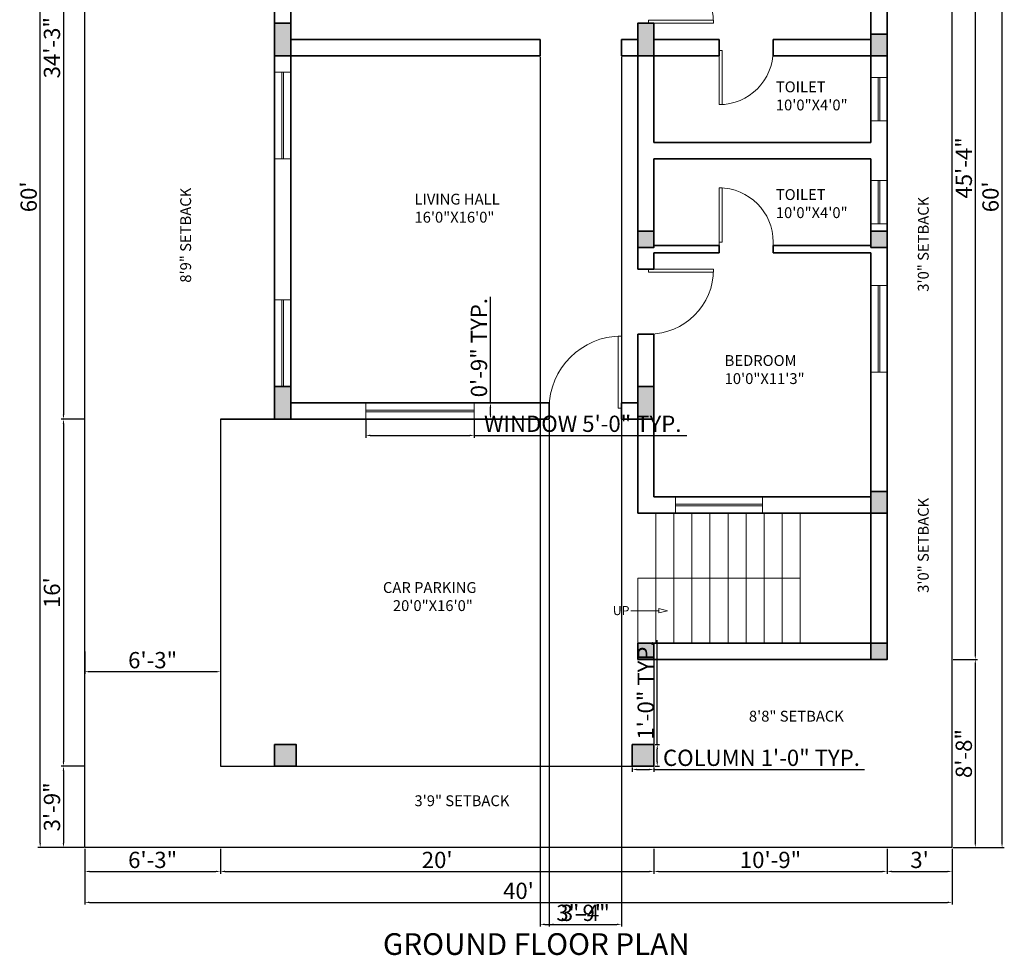
# Model space of a CAD drawing. Units: inches. Extents: x 3321 to 5237, y 11 to 1752.
# Tile 1 of 43: x 3321 to 3866, y 11 to 529. Entities that reach past the tile are written whole.
import ezdxf

# ---------------------------------------------------------------- set-up
doc = ezdxf.new("R2010")
doc.units = ezdxf.units.IN
for name, color, linetype, lineweight in [('A-ANNO-DIMS', 2, 'Continuous', 18), ('A-ANNO-SYMB', 7, 'Continuous', 18), ('A-ANNO-TEXT', 7, 'Continuous', 18), ('A-ANNO-TITL', 7, 'Continuous', 25), ('A-AREA-IDEN', 7, 'Continuous', 18), ('A-COLS', 1, 'Continuous', 35), ('A-DOOR', 4, 'Continuous', 18), ('A-FLOR-EDGE', 7, 'Continuous', 25), ('A-FLOR-STRS', 7, 'Continuous', 18), ('A-GLAZ', 5, 'Continuous', 18), ('A-WALL', 7, 'Continuous', 35), ('C-PROP', 7, 'Continuous', 30)]:
    doc.layers.add(name, color=color, linetype=linetype, lineweight=lineweight)
doc.styles.get("Standard").update_dxf_attribs({"font": 'arial.ttf'})
doc.dimstyles.new('ISO-25', dxfattribs={"dimtxt": 9, "dimasz": 2.5, "dimexe": 1.25, "dimexo": 0.625, "dimtad": 1, "dimdec": 1, "dimlunit": 3, "dimtxsty": 'Standard', "dimcen": 2.5, "dimclrd": 4, "dimclre": 4, "dimclrt": 256, "dimadec": 0, "dimazin": 0, "dimtfac": 1, "dimtdec": 1, "dimtmove": 0, "dimatfit": 3, "dimfxl": 1, "dimarcsym": 0})

# ---------------------------------------------------------------- blocks, each defined once
blk = doc.blocks.new('*U2')
for p, q in [((0, 0), (0, -6)), ((-40, 0), (-40, -6))]:
    blk.add_line(p, q)
blk.add_lwpolyline([(0, 0), (0, 40), (-1.75, 40), (-1.75, 0)], close=True)
blk.add_arc((0, 0), 40, 90, 180)
blk = doc.blocks.new('*U3')
for p, q in [((0, 0), (0, -6)), ((36, 0), (36, -6))]:
    blk.add_line(p, q)
blk.add_lwpolyline([(0, 0), (0, 36), (1.75, 36), (1.75, 0)], close=True)
blk.add_arc((0, 0), 36, 0, 90)
blk = doc.blocks.new('*U4')
for p, q in [((0, 0), (0, -6)), ((-36, 0), (-36, -6))]:
    blk.add_line(p, q)
blk.add_lwpolyline([(0, 0), (0, 36), (-1.75, 36), (-1.75, 0)], close=True)
blk.add_arc((0, 0), 36, 90, 180)
blk = doc.blocks.new('*U5')
for p, q in [((0, 0), (0, -6)), ((-30, 0), (-30, -6))]:
    blk.add_line(p, q)
blk.add_lwpolyline([(0, 0), (0, 30), (-1.75, 30), (-1.75, 0)], close=True)
blk.add_arc((0, 0), 30, 90, 180)
blk = doc.blocks.new('*U6')
for p, q in [((-30, 0), (-30, 6)), ((0, 0), (0, 6))]:
    blk.add_line(p, q)
blk.add_lwpolyline([(0, 0), (0, -30), (-1.75, -30), (-1.75, 0)], close=True)
blk.add_arc((0, 0), 30, 180, 270)
blk = doc.blocks.new('*D76')
at = {"layer": 'A-ANNO-DIMS', "color": 0, "lineweight": -2, "transparency": 16777216}
for p, q in [((3356.69, 179.02), (3356.69, 166.65)), ((3431.69, 179.02), (3431.69, 166.65)), ((3429.19, 167.9), (3359.19, 167.9))]:
    blk.add_line(p, q, dxfattribs=at)
at = {"layer": 'A-ANNO-DIMS', "color": 0, "transparency": 16777216}
for points in [[(3359.19, 168.32), (3359.19, 167.48), (3356.69, 167.9)], [(3429.19, 168.32), (3429.19, 167.48), (3431.69, 167.9)]]:
    blk.add_solid(points, dxfattribs=at)
at = {"layer": 'Defpoints', "color": 0, "transparency": 16777216}
for p in [(3356.69, 179.65), (3431.69, 179.65), (3356.69, 167.9)]:
    blk.add_point(p, dxfattribs=at)
at = {"layer": 'A-ANNO-DIMS', "color": 0, "transparency": 16777216, "insert": (3394.19, 173.12), "char_height": 9, "attachment_point": 5}
blk.add_mtext('6\'-3"', dxfattribs=at)
blk = doc.blocks.new('*D70')
at = {"layer": 'A-ANNO-DIMS', "color": 0, "lineweight": -2, "transparency": 16777216}
for p, q in [((3356.06, 718.61), (3343.59, 718.61)), ((3344.84, 716.11), (3344.84, 310.11)), ((3356.06, 307.61), (3343.59, 307.61))]:
    blk.add_line(p, q, dxfattribs=at)
at = {"layer": 'A-ANNO-DIMS', "color": 0, "transparency": 16777216}
for points in [[(3344.42, 716.11), (3345.26, 716.11), (3344.84, 718.61)], [(3344.42, 310.11), (3345.26, 310.11), (3344.84, 307.61)]]:
    blk.add_solid(points, dxfattribs=at)
at = {"layer": 'Defpoints', "color": 0, "transparency": 16777216}
for p in [(3356.69, 718.61), (3344.84, 307.61), (3356.69, 307.61)]:
    blk.add_point(p, dxfattribs=at)
at = {"layer": 'A-ANNO-DIMS', "color": 0, "transparency": 16777216, "insert": (3339.62, 513.11), "char_height": 9, "attachment_point": 5, "rotation": 90}
blk.add_mtext('34\'-3"', dxfattribs=at)
blk = doc.blocks.new('*D67')
at = {"layer": 'A-ANNO-DIMS', "color": 0, "lineweight": -2, "transparency": 16777216}
for p, q in [((3356.06, 307.61), (3343.59, 307.61)), ((3344.84, 305.11), (3344.84, 118.11)), ((3356.06, 115.61), (3343.59, 115.61))]:
    blk.add_line(p, q, dxfattribs=at)
at = {"layer": 'A-ANNO-DIMS', "color": 0, "transparency": 16777216}
for points in [[(3344.42, 305.11), (3345.26, 305.11), (3344.84, 307.61)], [(3344.42, 118.11), (3345.26, 118.11), (3344.84, 115.61)]]:
    blk.add_solid(points, dxfattribs=at)
at = {"layer": 'Defpoints', "color": 0, "transparency": 16777216}
for p in [(3356.69, 307.61), (3344.84, 115.61), (3356.69, 115.61)]:
    blk.add_point(p, dxfattribs=at)
at = {"layer": 'A-ANNO-DIMS', "color": 0, "transparency": 16777216, "insert": (3339.62, 211.61), "char_height": 9, "attachment_point": 5, "rotation": 90}
blk.add_mtext("16'", dxfattribs=at)
blk = doc.blocks.new('*D77')
at = {"layer": 'A-ANNO-DIMS', "color": 0, "lineweight": -2, "transparency": 16777216}
for p, q in [((3356.06, 115.61), (3343.59, 115.61)), ((3344.84, 113.11), (3344.84, 73.11)), ((3356.06, 70.61), (3343.59, 70.61))]:
    blk.add_line(p, q, dxfattribs=at)
at = {"layer": 'A-ANNO-DIMS', "color": 0, "transparency": 16777216}
for points in [[(3344.42, 113.11), (3345.26, 113.11), (3344.84, 115.61)], [(3344.42, 73.11), (3345.26, 73.11), (3344.84, 70.61)]]:
    blk.add_solid(points, dxfattribs=at)
at = {"layer": 'Defpoints', "color": 0, "transparency": 16777216}
for p in [(3356.69, 115.61), (3344.84, 70.61), (3356.69, 70.61)]:
    blk.add_point(p, dxfattribs=at)
at = {"layer": 'A-ANNO-DIMS', "color": 0, "transparency": 16777216, "insert": (3339.62, 93.11), "char_height": 9, "attachment_point": 5, "rotation": 90}
blk.add_mtext('3\'-9"', dxfattribs=at)
blk = doc.blocks.new('*D78')
at = {"layer": 'A-ANNO-DIMS', "color": 0, "lineweight": -2, "transparency": 16777216}
for p, q in [((3356.69, 69.98), (3356.69, 56.13)), ((3431.69, 69.98), (3431.69, 56.13)), ((3359.19, 57.38), (3429.19, 57.38))]:
    blk.add_line(p, q, dxfattribs=at)
at = {"layer": 'A-ANNO-DIMS', "color": 0, "transparency": 16777216}
for points in [[(3359.19, 57.8), (3359.19, 56.97), (3356.69, 57.38)], [(3429.19, 57.8), (3429.19, 56.97), (3431.69, 57.38)]]:
    blk.add_solid(points, dxfattribs=at)
at = {"layer": 'Defpoints', "color": 0, "transparency": 16777216}
for p in [(3356.69, 70.61), (3431.69, 70.61), (3431.69, 57.38)]:
    blk.add_point(p, dxfattribs=at)
at = {"layer": 'A-ANNO-DIMS', "color": 0, "transparency": 16777216, "insert": (3394.19, 62.61), "char_height": 9, "attachment_point": 5}
blk.add_mtext('6\'-3"', dxfattribs=at)
blk = doc.blocks.new('*D68')
at = {"layer": 'A-ANNO-DIMS', "color": 0, "lineweight": -2, "transparency": 16777216}
for p, q in [((3431.69, 69.98), (3431.69, 56.13)), ((3671.69, 69.98), (3671.69, 56.13)), ((3434.19, 57.38), (3669.19, 57.38))]:
    blk.add_line(p, q, dxfattribs=at)
at = {"layer": 'A-ANNO-DIMS', "color": 0, "transparency": 16777216}
for points in [[(3434.19, 57.8), (3434.19, 56.97), (3431.69, 57.38)], [(3669.19, 57.8), (3669.19, 56.97), (3671.69, 57.38)]]:
    blk.add_solid(points, dxfattribs=at)
at = {"layer": 'Defpoints', "color": 0, "transparency": 16777216}
for p in [(3431.69, 70.61), (3671.69, 70.61), (3671.69, 57.38)]:
    blk.add_point(p, dxfattribs=at)
at = {"layer": 'A-ANNO-DIMS', "color": 0, "transparency": 16777216, "insert": (3551.69, 62.6), "char_height": 9, "attachment_point": 5}
blk.add_mtext("20'", dxfattribs=at)
blk = doc.blocks.new('*D69')
at = {"layer": 'A-ANNO-DIMS', "color": 0, "lineweight": -2, "transparency": 16777216}
for p, q in [((3671.69, 69.98), (3671.69, 56.13)), ((3800.69, 69.98), (3800.69, 56.13)), ((3674.19, 57.38), (3798.19, 57.38))]:
    blk.add_line(p, q, dxfattribs=at)
at = {"layer": 'A-ANNO-DIMS', "color": 0, "transparency": 16777216}
for points in [[(3674.19, 57.8), (3674.19, 56.97), (3671.69, 57.38)], [(3798.19, 57.8), (3798.19, 56.97), (3800.69, 57.38)]]:
    blk.add_solid(points, dxfattribs=at)
at = {"layer": 'Defpoints', "color": 0, "transparency": 16777216}
for p in [(3671.69, 70.61), (3800.69, 70.61), (3800.69, 57.38)]:
    blk.add_point(p, dxfattribs=at)
at = {"layer": 'A-ANNO-DIMS', "color": 0, "transparency": 16777216, "insert": (3736.19, 62.6), "char_height": 9, "attachment_point": 5}
blk.add_mtext('10\'-9"', dxfattribs=at)
blk = doc.blocks.new('*D80')
at = {"layer": 'A-ANNO-DIMS', "color": 0, "lineweight": -2, "transparency": 16777216}
for p, q in [((3800.69, 69.98), (3800.69, 56.13)), ((3836.69, 69.98), (3836.69, 56.13)), ((3803.19, 57.38), (3834.19, 57.38))]:
    blk.add_line(p, q, dxfattribs=at)
at = {"layer": 'A-ANNO-DIMS', "color": 0, "transparency": 16777216}
for points in [[(3803.19, 57.8), (3803.19, 56.97), (3800.69, 57.38)], [(3834.19, 57.8), (3834.19, 56.97), (3836.69, 57.38)]]:
    blk.add_solid(points, dxfattribs=at)
at = {"layer": 'Defpoints', "color": 0, "transparency": 16777216}
for p in [(3800.69, 70.61), (3836.69, 70.61), (3836.69, 57.38)]:
    blk.add_point(p, dxfattribs=at)
at = {"layer": 'A-ANNO-DIMS', "color": 0, "transparency": 16777216, "insert": (3818.69, 62.61), "char_height": 9, "attachment_point": 5}
blk.add_mtext("3'", dxfattribs=at)
blk = doc.blocks.new('*D74')
at = {"layer": 'A-ANNO-DIMS', "color": 0, "lineweight": -2, "transparency": 16777216}
for p, q in [((3837.31, 718.61), (3850.8, 718.61)), ((3849.55, 716.11), (3849.55, 177.11)), ((3837.31, 174.61), (3850.8, 174.61))]:
    blk.add_line(p, q, dxfattribs=at)
at = {"layer": 'A-ANNO-DIMS', "color": 0, "transparency": 16777216}
for points in [[(3849.13, 716.11), (3849.96, 716.11), (3849.55, 718.61)], [(3849.13, 177.11), (3849.96, 177.11), (3849.55, 174.61)]]:
    blk.add_solid(points, dxfattribs=at)
at = {"layer": 'Defpoints', "color": 0, "transparency": 16777216}
for p in [(3836.69, 718.61), (3836.69, 174.61), (3849.55, 174.61)]:
    blk.add_point(p, dxfattribs=at)
at = {"layer": 'A-ANNO-DIMS', "color": 0, "transparency": 16777216, "insert": (3844.35, 446.61), "char_height": 9, "attachment_point": 5, "rotation": 90}
blk.add_mtext('45\'-4"', dxfattribs=at)
blk = doc.blocks.new('*D75')
at = {"layer": 'A-ANNO-DIMS', "color": 0, "lineweight": -2, "transparency": 16777216}
for p, q in [((3837.31, 174.61), (3850.8, 174.61)), ((3849.55, 172.11), (3849.55, 73.11)), ((3837.31, 70.61), (3850.8, 70.61))]:
    blk.add_line(p, q, dxfattribs=at)
at = {"layer": 'A-ANNO-DIMS', "color": 0, "transparency": 16777216}
for points in [[(3849.13, 172.11), (3849.96, 172.11), (3849.55, 174.61)], [(3849.13, 73.11), (3849.96, 73.11), (3849.55, 70.61)]]:
    blk.add_solid(points, dxfattribs=at)
at = {"layer": 'Defpoints', "color": 0, "transparency": 16777216}
for p in [(3836.69, 174.61), (3836.69, 70.61), (3849.55, 70.61)]:
    blk.add_point(p, dxfattribs=at)
at = {"layer": 'A-ANNO-DIMS', "color": 0, "transparency": 16777216, "insert": (3844.33, 122.61), "char_height": 9, "attachment_point": 5, "rotation": 90}
blk.add_mtext('8\'-8"', dxfattribs=at)
blk = doc.blocks.new('*D83')
at = {"layer": 'A-ANNO-DIMS', "color": 0, "lineweight": -2, "transparency": 16777216}
for p, q in [((3356.06, 790.61), (3330.71, 790.61)), ((3331.96, 73.11), (3331.96, 788.11)), ((3356.06, 70.61), (3330.71, 70.61))]:
    blk.add_line(p, q, dxfattribs=at)
at = {"layer": 'A-ANNO-DIMS', "color": 0, "transparency": 16777216}
for points in [[(3331.55, 788.11), (3332.38, 788.11), (3331.96, 790.61)], [(3331.55, 73.11), (3332.38, 73.11), (3331.96, 70.61)]]:
    blk.add_solid(points, dxfattribs=at)
at = {"layer": 'Defpoints', "color": 0, "transparency": 16777216}
for p in [(3331.96, 790.61), (3356.69, 790.61), (3356.69, 70.61)]:
    blk.add_point(p, dxfattribs=at)
at = {"layer": 'A-ANNO-DIMS', "color": 0, "transparency": 16777216, "insert": (3326.74, 430.61), "char_height": 9, "attachment_point": 5, "rotation": 90}
blk.add_mtext("60'", dxfattribs=at)
blk = doc.blocks.new('*D84')
at = {"layer": 'A-ANNO-DIMS', "color": 0, "lineweight": -2, "transparency": 16777216}
for p, q in [((3356.69, 69.98), (3356.69, 39.03)), ((3836.69, 69.98), (3836.69, 39.03)), ((3359.19, 40.28), (3834.19, 40.28))]:
    blk.add_line(p, q, dxfattribs=at)
at = {"layer": 'A-ANNO-DIMS', "color": 0, "transparency": 16777216}
for points in [[(3359.19, 40.7), (3359.19, 39.86), (3356.69, 40.28)], [(3834.19, 40.7), (3834.19, 39.86), (3836.69, 40.28)]]:
    blk.add_solid(points, dxfattribs=at)
at = {"layer": 'Defpoints', "color": 0, "transparency": 16777216}
for p in [(3356.69, 70.61), (3836.69, 70.61), (3836.69, 40.28)]:
    blk.add_point(p, dxfattribs=at)
at = {"layer": 'A-ANNO-DIMS', "color": 0, "transparency": 16777216, "insert": (3596.69, 45.5), "char_height": 9, "attachment_point": 5}
blk.add_mtext("40'", dxfattribs=at)
blk = doc.blocks.new('*D85')
at = {"layer": 'A-ANNO-DIMS', "color": 0, "lineweight": -2, "transparency": 16777216}
for p, q in [((3837.31, 790.61), (3865.6, 790.61)), ((3864.35, 73.11), (3864.35, 788.11)), ((3837.31, 70.61), (3865.6, 70.61))]:
    blk.add_line(p, q, dxfattribs=at)
at = {"layer": 'A-ANNO-DIMS', "color": 0, "transparency": 16777216}
for points in [[(3863.93, 788.11), (3864.76, 788.11), (3864.35, 790.61)], [(3863.93, 73.11), (3864.76, 73.11), (3864.35, 70.61)]]:
    blk.add_solid(points, dxfattribs=at)
at = {"layer": 'Defpoints', "color": 0, "transparency": 16777216}
for p in [(3836.69, 790.61), (3864.35, 790.61), (3836.69, 70.61)]:
    blk.add_point(p, dxfattribs=at)
at = {"layer": 'A-ANNO-DIMS', "color": 0, "transparency": 16777216, "insert": (3859.13, 430.61), "char_height": 9, "attachment_point": 5, "rotation": 90}
blk.add_mtext("60'", dxfattribs=at)
blk = doc.blocks.new('COL-9X18-IN')
h = blk.add_hatch(color=256)
h.dxf.hatch_style = 1
h.paths.add_polyline_path([(9, 18), (0, 18), (0, 0), (9, 0)])
blk.add_lwpolyline([(0, 0), (9, 0), (9, 18), (0, 18)], close=True)
blk = doc.blocks.new('COL-9X12-BASE-PLAN')
h = blk.add_hatch(color=256)
h.dxf.hatch_style = 1
h.paths.add_polyline_path([(0, 0), (9, 0), (9, 12), (0, 12)])
blk.add_lwpolyline([(0, 0), (9, 0), (9, 12), (0, 12)], close=True)
blk = doc.blocks.new('COL-9X9-BASE-PLAN')
h = blk.add_hatch(color=256)
h.dxf.hatch_style = 1
h.paths.add_polyline_path([(0, 0), (9, 0), (9, 9), (0, 9)])
blk.add_lwpolyline([(0, 0), (9, 0), (9, 9), (0, 9)], close=True)
blk = doc.blocks.new('COL-12X12-BASE-PLAN')
h = blk.add_hatch(color=256)
h.dxf.hatch_style = 1
h.paths.add_polyline_path([(0, 0), (12, 0), (12, 12), (0, 12)])
blk.add_lwpolyline([(0, 0), (12, 0), (12, 12), (0, 12)], close=True)
blk = doc.blocks.new('WIN-48IN-9IN-WALL')
for p, q in [((0, 0), (0, 9)), ((48, 0), (48, 9)), ((0, 5), (48, 5)), ((0, 4), (48, 4))]:
    blk.add_line(p, q)
blk = doc.blocks.new('WIN-60IN-9IN-WALL')
for p, q in [((0, 0), (0, 9)), ((60, 0), (60, 9)), ((0, 5), (60, 5)), ((0, 4), (60, 4))]:
    blk.add_line(p, q)
blk = doc.blocks.new('WIN-24IN-9IN-WALL')
for p, q in [((9, 24), (0, 24)), ((4, 24), (4, 0)), ((5, 24), (5, 0)), ((9, 0), (0, 0))]:
    blk.add_line(p, q)
blk = doc.blocks.new('STAIR-RETURN-72IN')
for p, q in [((10, 72), (10, 0)), ((20, 72), (20, 0)), ((30, 72), (30, 0)), ((40, 72), (40, 0)), ((50, 72), (50, 0)), ((60, 72), (60, 0)), ((70, 72), (70, 0)), ((80, 72), (80, 0)), ((90, 72), (90, 0)), ((90, 36), (0, 36)), ((0, 36), (0, 0))]:
    blk.add_line(p, q)
blk = doc.blocks.new('STAIR-DIRECTION-ARROW')
blk.add_line((0, 1.22), (15.43, 1.22))
blk.add_lwpolyline([(20.27, 1.22), (15.43, 2.43), (15.43, 0)], close=True)
blk = doc.blocks.new('PROPERTY-40X60FT')
for p, q in [((0, 720), (480, 720)), ((0, 720), (0, 0)), ((480, 720), (480, 0)), ((0, 0), (480, 0))]:
    blk.add_line(p, q)
blk = doc.blocks.new('*D171')
at = {"layer": 'A-ANNO-DIMS', "color": 4, "lineweight": -2, "transparency": 16777216}
for p, q in [((3512.19, 306.98), (3512.19, 297.36)), ((3572.19, 306.98), (3572.19, 297.36)), ((3514.69, 298.61), (3569.69, 298.61)), ((3572.19, 298.61), (3689.83, 298.61))]:
    blk.add_line(p, q, dxfattribs=at)
at = {"layer": 'A-ANNO-DIMS', "color": 4, "transparency": 16777216}
for points in [[(3514.69, 299.02), (3514.69, 298.19), (3512.19, 298.61)], [(3569.69, 299.02), (3569.69, 298.19), (3572.19, 298.61)]]:
    blk.add_solid(points, dxfattribs=at)
at = {"layer": 'Defpoints', "color": 0, "transparency": 16777216}
for p in [(3512.19, 307.61), (3572.19, 307.61), (3572.19, 298.61)]:
    blk.add_point(p, dxfattribs=at)
at = {"layer": 'A-ANNO-DIMS', "transparency": 16777216, "insert": (3632.26, 303.89), "char_height": 9, "attachment_point": 5}
blk.add_mtext('WINDOW 5\'-0" TYP.', dxfattribs=at)
blk = doc.blocks.new('*D172')
at = {"layer": 'A-ANNO-DIMS', "color": 4, "lineweight": -2, "transparency": 16777216}
for p, q in [((3581.19, 316.61), (3581.19, 375.22)), ((3572.81, 316.61), (3582.44, 316.61)), ((3581.19, 310.11), (3581.19, 314.11)), ((3572.81, 307.61), (3582.44, 307.61))]:
    blk.add_line(p, q, dxfattribs=at)
at = {"layer": 'A-ANNO-DIMS', "color": 4, "transparency": 16777216}
for points in [[(3580.77, 314.11), (3581.61, 314.11), (3581.19, 316.61)], [(3580.77, 310.11), (3581.61, 310.11), (3581.19, 307.61)]]:
    blk.add_solid(points, dxfattribs=at)
at = {"layer": 'Defpoints', "color": 0, "transparency": 16777216}
for p in [(3572.19, 316.61), (3581.19, 316.61), (3572.19, 307.61)]:
    blk.add_point(p, dxfattribs=at)
at = {"layer": 'A-ANNO-DIMS', "transparency": 16777216, "insert": (3575.97, 347.16), "char_height": 9, "attachment_point": 5, "rotation": 90}
blk.add_mtext('0\'-9" TYP.', dxfattribs=at)
blk = doc.blocks.new('*D183')
at = {"layer": 'A-ANNO-DIMS', "color": 4, "lineweight": -2, "transparency": 16777216}
for p, q in [((3659.69, 114.98), (3659.69, 112.56)), ((3671.69, 114.98), (3671.69, 112.56)), ((3662.19, 113.81), (3669.19, 113.81)), ((3671.69, 113.81), (3788.17, 113.81))]:
    blk.add_line(p, q, dxfattribs=at)
at = {"layer": 'A-ANNO-DIMS', "color": 4, "transparency": 16777216}
for points in [[(3662.19, 114.22), (3662.19, 113.39), (3659.69, 113.81)], [(3669.19, 114.22), (3669.19, 113.39), (3671.69, 113.81)]]:
    blk.add_solid(points, dxfattribs=at)
at = {"layer": 'Defpoints', "color": 0, "transparency": 16777216}
for p in [(3659.69, 115.61), (3671.69, 115.61), (3671.69, 113.81)]:
    blk.add_point(p, dxfattribs=at)
at = {"layer": 'A-ANNO-DIMS', "transparency": 16777216, "insert": (3731.18, 119.09), "char_height": 9, "attachment_point": 5}
blk.add_mtext('COLUMN 1\'-0" TYP.', dxfattribs=at)
blk = doc.blocks.new('*D184')
at = {"layer": 'A-ANNO-DIMS', "color": 4, "lineweight": -2, "transparency": 16777216}
for p, q in [((3673.49, 127.61), (3673.49, 185.37)), ((3672.31, 127.61), (3674.74, 127.61)), ((3673.49, 118.11), (3673.49, 125.11)), ((3672.31, 115.61), (3674.74, 115.61))]:
    blk.add_line(p, q, dxfattribs=at)
at = {"layer": 'A-ANNO-DIMS', "color": 4, "transparency": 16777216}
for points in [[(3673.07, 125.11), (3673.91, 125.11), (3673.49, 127.61)], [(3673.07, 118.11), (3673.91, 118.11), (3673.49, 115.61)]]:
    blk.add_solid(points, dxfattribs=at)
at = {"layer": 'Defpoints', "color": 0, "transparency": 16777216}
for p in [(3671.69, 127.61), (3673.49, 127.61), (3671.69, 115.61)]:
    blk.add_point(p, dxfattribs=at)
at = {"layer": 'A-ANNO-DIMS', "transparency": 16777216, "insert": (3668.27, 157.74), "char_height": 9, "attachment_point": 5, "rotation": 90}
blk.add_mtext('1\'-0" TYP.', dxfattribs=at)
blk = doc.blocks.new('*D223')
at = {"layer": 'A-ANNO-DIMS', "color": 4, "lineweight": -2, "transparency": 16777216}
for p, q in [((3613.69, 306.98), (3613.69, 26.86)), ((3653.69, 306.98), (3653.69, 26.86)), ((3616.19, 28.11), (3651.19, 28.11))]:
    blk.add_line(p, q, dxfattribs=at)
at = {"layer": 'A-ANNO-DIMS', "color": 4, "transparency": 16777216}
for points in [[(3616.19, 28.52), (3616.19, 27.69), (3613.69, 28.11)], [(3651.19, 28.52), (3651.19, 27.69), (3653.69, 28.11)]]:
    blk.add_solid(points, dxfattribs=at)
at = {"layer": 'Defpoints', "color": 0, "transparency": 16777216}
for p in [(3613.69, 307.61), (3653.69, 307.61), (3653.69, 28.11)]:
    blk.add_point(p, dxfattribs=at)
at = {"layer": 'A-ANNO-DIMS', "transparency": 16777216, "insert": (3633.69, 33.33), "char_height": 9, "attachment_point": 5}
blk.add_mtext('3\'-4"', dxfattribs=at)
blk = doc.blocks.new('*D224')
at = {"layer": 'A-ANNO-DIMS', "color": 4, "lineweight": -2, "transparency": 16777216}
for p, q in [((3608.69, 507.98), (3608.69, 26.86)), ((3653.69, 507.98), (3653.69, 26.86)), ((3611.19, 28.11), (3651.19, 28.11))]:
    blk.add_line(p, q, dxfattribs=at)
at = {"layer": 'A-ANNO-DIMS', "color": 4, "transparency": 16777216}
for points in [[(3611.19, 28.52), (3611.19, 27.69), (3608.69, 28.11)], [(3651.19, 28.52), (3651.19, 27.69), (3653.69, 28.11)]]:
    blk.add_solid(points, dxfattribs=at)
at = {"layer": 'Defpoints', "color": 0, "transparency": 16777216}
for p in [(3608.69, 508.61), (3653.69, 508.61), (3653.69, 28.11)]:
    blk.add_point(p, dxfattribs=at)
at = {"layer": 'A-ANNO-DIMS', "transparency": 16777216, "insert": (3631.19, 33.33), "char_height": 9, "attachment_point": 5}
blk.add_mtext('3\'-9"', dxfattribs=at)

msp = doc.modelspace()

# ---------------------------------------------------------------- linework, layer by layer
at = {"layer": 'A-FLOR-EDGE'}
for p, q in [((3431.69, 307.61), (3431.69, 115.61)), ((3671.69, 174.61), (3671.69, 115.61)), ((3431.69, 115.61), (3671.69, 115.61))]:
    msp.add_line(p, q, dxfattribs=at)
at = {"layer": 'A-WALL'}
for p, q in [((3461.69, 718.61), (3461.69, 307.61)), ((3800.69, 718.61), (3800.69, 174.61)), ((3791.69, 709.61), (3791.69, 517.61)), ((3470.69, 609.61), (3470.69, 517.61)), ((3662.69, 526.61), (3662.69, 517.61)), ((3662.69, 526.61), (3671.69, 526.61)), ((3671.69, 526.61), (3671.69, 517.61)), ((3470.69, 517.61), (3608.69, 517.61)), ((3608.69, 517.61), (3608.69, 508.61)), ((3653.69, 517.61), (3662.69, 517.61)), ((3653.69, 517.61), (3653.69, 508.61)), ((3671.69, 517.61), (3707.69, 517.61)), ((3707.69, 508.61), (3707.69, 517.61)), ((3737.69, 517.61), (3791.69, 517.61)), ((3737.69, 508.61), (3737.69, 517.61)), ((3470.69, 508.61), (3470.69, 316.61)), ((3470.69, 508.61), (3608.69, 508.61)), ((3653.69, 508.61), (3662.69, 508.61)), ((3662.69, 508.61), (3662.69, 390.61)), ((3671.69, 508.61), (3671.69, 460.61)), ((3671.69, 508.61), (3707.69, 508.61)), ((3737.69, 508.61), (3791.69, 508.61)), ((3791.69, 508.61), (3791.69, 460.61)), ((3671.69, 460.61), (3791.69, 460.61)), ((3671.69, 451.61), (3671.69, 403.61)), ((3671.69, 451.61), (3791.69, 451.61)), ((3791.69, 451.61), (3791.69, 403.61)), ((3671.69, 403.61), (3707.69, 403.61)), ((3707.69, 403.61), (3707.69, 399.61)), ((3737.69, 403.61), (3791.69, 403.61)), ((3737.69, 403.61), (3737.69, 399.61)), ((3671.69, 399.61), (3671.69, 390.61)), ((3671.69, 399.61), (3707.69, 399.61)), ((3737.69, 399.61), (3791.69, 399.61)), ((3791.69, 399.61), (3791.69, 264.61)), ((3662.69, 390.61), (3671.69, 390.61)), ((3662.69, 354.61), (3662.69, 316.61)), ((3662.69, 354.61), (3671.69, 354.61)), ((3671.69, 354.61), (3671.69, 264.61)), ((3470.69, 316.61), (3613.69, 316.61)), ((3613.69, 316.61), (3613.69, 307.61)), ((3653.69, 316.61), (3662.69, 316.61)), ((3653.69, 316.61), (3653.69, 307.61)), ((3431.69, 307.61), (3613.69, 307.61)), ((3653.69, 307.61), (3662.69, 307.61)), ((3662.69, 307.61), (3662.69, 255.61)), ((3671.69, 264.61), (3791.69, 264.61)), ((3662.69, 255.61), (3791.69, 255.61)), ((3791.69, 255.61), (3791.69, 183.61)), ((3662.69, 183.61), (3662.69, 174.61)), ((3662.69, 183.61), (3791.69, 183.61)), ((3662.69, 174.61), (3800.69, 174.61))]:
    msp.add_line(p, q, dxfattribs=at)

# ---------------------------------------------------------------- block references
at = {"layer": 'A-ANNO-SYMB'}
msp.add_blockref('STAIR-DIRECTION-ARROW', (3658.96, 200.39), dxfattribs=at)
at = {"layer": 'A-COLS', "rotation": 180}
for p in [(3470.69, 526.61), (3671.69, 526.61), (3470.69, 325.61), (3671.69, 325.61)]:
    msp.add_blockref('COL-9X18-IN', p, dxfattribs=at)
at = {"layer": 'A-COLS'}
for name, p in [('COL-9X12-BASE-PLAN', (3791.69, 508.61)), ('COL-9X9-BASE-PLAN', (3662.69, 402.61)), ('COL-9X9-BASE-PLAN', (3791.69, 402.61)), ('COL-9X12-BASE-PLAN', (3791.69, 255.61)), ('COL-9X9-BASE-PLAN', (3662.69, 174.61)), ('COL-9X9-BASE-PLAN', (3791.69, 174.61)), ('COL-12X12-BASE-PLAN', (3461.69, 115.61)), ('COL-12X12-BASE-PLAN', (3659.69, 115.61))]:
    msp.add_blockref(name, p, dxfattribs=at)
at = {"layer": 'A-DOOR'}
for name, p, rotation in [('*U4', (3668.69, 526.61), 270), ('*U5', (3707.69, 511.61), 180), ('*U6', (3707.69, 405.61), 180), ('*U3', (3668.69, 390.61), 270)]:
    msp.add_blockref(name, p, dxfattribs=dict(at, rotation=rotation))
msp.add_blockref('*U2', (3653.69, 313.61), dxfattribs=at)
at = {"layer": 'A-FLOR-STRS'}
msp.add_blockref('STAIR-RETURN-72IN', (3662.69, 183.61), dxfattribs=at)
at = {"layer": 'A-GLAZ'}
for p, rotation in [((3470.69, 451.61), 89.99999999999824), ((3800.69, 333.61), 89.9999999999993), ((3470.69, 325.61), 89.99999999999824)]:
    msp.add_blockref('WIN-48IN-9IN-WALL', p, dxfattribs=dict(at, rotation=rotation))
for name, p in [('WIN-24IN-9IN-WALL', (3791.69, 472.61)), ('WIN-24IN-9IN-WALL', (3791.69, 415.61)), ('WIN-60IN-9IN-WALL', (3512.19, 307.61)), ('WIN-48IN-9IN-WALL', (3683.69, 255.61))]:
    msp.add_blockref(name, p, dxfattribs=at)
at = {"layer": 'C-PROP', "rotation": 180}
msp.add_blockref('PROPERTY-40X60FT', (3836.69, 790.61), dxfattribs=at)

# ---------------------------------------------------------------- texts
at = {"layer": 'A-ANNO-TEXT'}
msp.add_text('UP', height=5, dxfattribs=at).set_placement((3648.91, 199.21))
at = {"layer": 'A-ANNO-TEXT', "char_height": 6, "attachment_point": 1, "rotation": 90}
for s, insert in [('8\'9" SETBACK', (3409.48, 383.1)), ('3\'0" SETBACK', (3817.76, 378.11)), ('3\'0" SETBACK', (3817.76, 211.53))]:
    msp.add_mtext_dynamic_manual_height_columns(s, width=97.3114, gutter_width=25, heights=[0], dxfattribs=dict(at, insert=insert))
at = {"layer": 'A-ANNO-TEXT', "char_height": 6, "attachment_point": 1}
for s, insert in [('8\'8" SETBACK', (3724.23, 146.28)), ('3\'9" SETBACK', (3539.12, 99.5))]:
    msp.add_mtext_dynamic_manual_height_columns(s, width=97.3114, gutter_width=25, heights=[0], dxfattribs=dict(at, insert=insert))
at = {"layer": 'A-ANNO-TITL', "insert": (3521.67, 23.21), "char_height": 12, "attachment_point": 1}
msp.add_mtext_dynamic_manual_height_columns('GROUND FLOOR PLAN', width=241.3793, gutter_width=25, heights=[0], dxfattribs=at)
at = {"layer": 'A-AREA-IDEN', "char_height": 6, "attachment_point": 1}
for s, width, insert in [('TOILET\\P10\'0"X4\'0"', 97.3114, (3739.14, 494.44)), ('LIVING HALL\\P16\'0"X16\'0"', 97.3114, (3539.12, 432.33)), ('TOILET\\P10\'0"X4\'0"', 97.3114, (3739.14, 434.86)), ('BEDROOM\\P10\'0"X11\'3"', 97.3114, (3710.8, 343.05)), ('CAR PARKING\\P   20\'0"X16\'0"', 108.2268, (3521.67, 217.46))]:
    msp.add_mtext_dynamic_manual_height_columns(s, width=width, gutter_width=25, heights=[0], dxfattribs=dict(at, insert=insert))

# ---------------------------------------------------------------- dimensions: what is measured, and where the dimension line sits
at = {"layer": 'A-ANNO-DIMS'}
for base, p1, p2, angle, override, picture, middle in [((3331.96, 790.61), (3356.69, 70.61), (3356.69, 790.61), 270, {"dimclrd": 0, "dimclre": 0, "dimclrt": 0}, '*D83', (3326.74, 430.61)), ((3864.35, 790.61), (3836.69, 70.61), (3836.69, 790.61), 270, {"dimclrd": 0, "dimclre": 0, "dimclrt": 0}, '*D85', (3859.13, 430.61)), ((3344.84, 307.61), (3356.69, 718.61), (3356.69, 307.61), 90, {"dimclrd": 0, "dimclre": 0, "dimclrt": 0, "dimtmove": 1}, '*D70', (3339.62, 513.11)), ((3849.55, 174.61), (3836.69, 718.61), (3836.69, 174.61), 90, {"dimclrd": 0, "dimclre": 0, "dimclrt": 0, "dimtmove": 1}, '*D74', (3844.35, 446.61)), ((3344.84, 115.61), (3356.69, 307.61), (3356.69, 115.61), 90, {"dimclrd": 0, "dimclre": 0, "dimclrt": 0, "dimtmove": 1}, '*D67', (3339.62, 211.61)), ((3849.55, 70.61), (3836.69, 174.61), (3836.69, 70.61), 90, {"dimclrd": 0, "dimclre": 0, "dimclrt": 0, "dimtmove": 1}, '*D75', (3844.33, 122.61)), ((3344.84, 70.61), (3356.69, 115.61), (3356.69, 70.61), 90, {"dimclrd": 0, "dimclre": 0, "dimclrt": 0, "dimtmove": 1}, '*D77', (3339.62, 93.11))]:
    dim = msp.add_linear_dim(base=base, p1=p1, p2=p2, angle=angle, dimstyle='ISO-25', override=override, dxfattribs=at)
    dim.commit()
    dim.dimension.update_dxf_attribs({"geometry": picture, "text_midpoint": middle})
for base, p1, p2, override, picture, middle in [((3653.69, 28.11), (3608.69, 508.61), (3653.69, 508.61), {"dimdec": 1, "dimlfac": 1, "dimrnd": 0, "dimzin": 1, "dimdsep": 46, "dimlunit": 4, "dimfrac": 2}, '*D224', (3631.19, 33.33)), ((3653.69, 28.11), (3613.69, 307.61), (3653.69, 307.61), {"dimdec": 1, "dimlfac": 1, "dimrnd": 0, "dimzin": 1, "dimdsep": 46, "dimlunit": 4, "dimfrac": 2}, '*D223', (3633.69, 33.33)), ((3356.69, 167.9), (3431.69, 179.65), (3356.69, 179.65), {"dimclrd": 0, "dimclre": 0, "dimclrt": 0}, '*D76', (3394.19, 173.12)), ((3431.69, 57.38), (3356.69, 70.61), (3431.69, 70.61), {"dimclrd": 0, "dimclre": 0, "dimclrt": 0}, '*D78', (3394.19, 62.61)), ((3836.69, 40.28), (3356.69, 70.61), (3836.69, 70.61), {"dimclrd": 0, "dimclre": 0, "dimclrt": 0}, '*D84', (3596.69, 45.5)), ((3671.69, 57.38), (3431.69, 70.61), (3671.69, 70.61), {"dimclrd": 0, "dimclre": 0, "dimclrt": 0, "dimtmove": 1}, '*D68', (3551.69, 62.6)), ((3800.69, 57.38), (3671.69, 70.61), (3800.69, 70.61), {"dimclrd": 0, "dimclre": 0, "dimclrt": 0, "dimtmove": 1}, '*D69', (3736.19, 62.6)), ((3836.69, 57.38), (3800.69, 70.61), (3836.69, 70.61), {"dimclrd": 0, "dimclre": 0, "dimclrt": 0, "dimtmove": 1}, '*D80', (3818.69, 62.61))]:
    dim = msp.add_linear_dim(base=base, p1=p1, p2=p2, dimstyle='ISO-25', override=override, dxfattribs=at)
    dim.commit()
    dim.dimension.update_dxf_attribs({"geometry": picture, "text_midpoint": middle})
for base, p1, p2, picture, middle in [((3581.19, 316.61), (3572.19, 307.61), (3572.19, 316.61), '*D172', (3575.97, 347.16)), ((3673.49, 127.61), (3671.69, 115.61), (3671.69, 127.61), '*D184', (3668.27, 157.74))]:
    dim = msp.add_linear_dim(base=base, p1=p1, p2=p2, angle=90, text='<> TYP.', dimstyle='ISO-25', override={"dimdec": 1, "dimlfac": 1, "dimrnd": 0, "dimzin": 1, "dimdsep": 46, "dimlunit": 4, "dimfrac": 2}, dxfattribs=at)
    dim.commit()
    dim.dimension.update_dxf_attribs({"geometry": picture, "text_midpoint": middle})
for base, p1, p2, text, picture, middle in [((3572.19, 298.61), (3512.19, 307.61), (3572.19, 307.61), 'WINDOW <> TYP.', '*D171', (3632.26, 303.89)), ((3671.69, 113.81), (3659.69, 115.61), (3671.69, 115.61), 'COLUMN <> TYP.', '*D183', (3731.18, 119.09))]:
    dim = msp.add_linear_dim(base=base, p1=p1, p2=p2, text=text, dimstyle='ISO-25', override={"dimdec": 1, "dimlfac": 1, "dimrnd": 0, "dimzin": 1, "dimdsep": 46, "dimlunit": 4, "dimfrac": 2}, dxfattribs=at)
    dim.commit()
    dim.dimension.update_dxf_attribs({"geometry": picture, "text_midpoint": middle})

doc.saveas('drawing.dxf')
